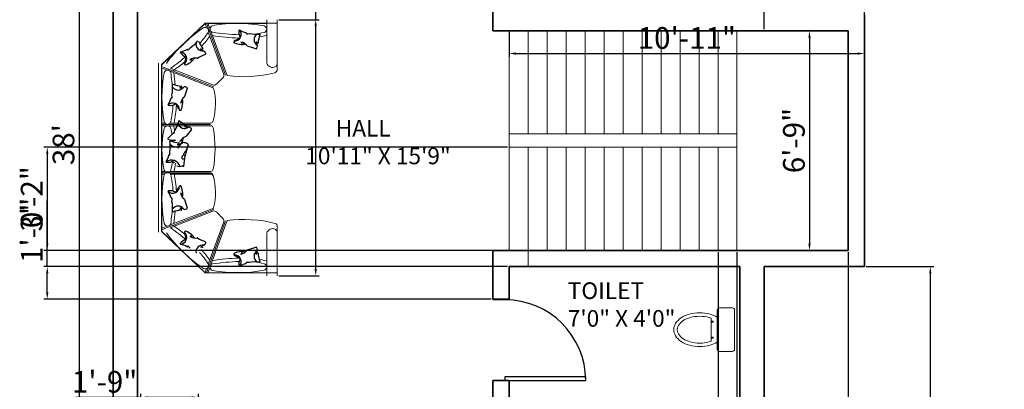
# Model space of a CAD drawing. Units: inches. Extents: x 3064 to 3427, y 2432 to 3115.
# Tile 2 of 3: x 3064 to 3427, y 2696 to 2833. Entities that reach past the tile are written whole.
import ezdxf

# ---------------------------------------------------------------- set-up
doc = ezdxf.new("R2010")
doc.units = ezdxf.units.IN
for name, color, linetype, lineweight in [('A-ANNO-DIMS', 2, 'Continuous', 13), ('A-AREA-IDEN', 7, 'Continuous', 18), ('A-DOOR', 4, 'Continuous', 25), ('A-FLOR-STRS', 3, 'Continuous', 18), ('A-WALL', 7, 'Continuous', 35), ('FUR', 42, 'Continuous', 18), ('THIET-BI', 21, 'Continuous', 18)]:
    doc.layers.add(name, color=color, linetype=linetype, lineweight=lineweight)
doc.layers.add('HID', color=11, linetype='Continuous')
doc.styles.get("Standard").update_dxf_attribs({"font": 'arial.ttf'})
doc.dimstyles.new('ISO-25', dxfattribs={"dimtxt": 8, "dimasz": 2.5, "dimexe": 1.25, "dimexo": 0.625, "dimtad": 1, "dimdec": 0, "dimlunit": 4, "dimtxsty": 'Standard', "dimcen": 2.5, "dimadec": 0, "dimazin": 0, "dimtfac": 1, "dimtdec": 0, "dimtmove": 0, "dimatfit": 3, "dimfxl": 1, "dimarcsym": 0})

# ---------------------------------------------------------------- blocks, each defined once
blk = doc.blocks.new('A$C5B9B1B1E')
at = {"layer": 'FUR'}
for p, q in [((0.68, 1.857), (3.32, 1.857)), ((0.044, 1.127), (0.687, 1.804)), ((0.046, 1.126), (0.691, 1.805)), ((0.687, 1.804), (3.246, 1.804)), ((0.689, 1.807), (3.298, 1.807)), ((0.718, 1.807), (1.035, 0.991)), ((0.741, 1.807), (0.774, 1.719)), ((1.587, 1.804), (1.587, 1.757)), ((1.608, 1.804), (1.608, 1.041)), ((1.629, 1.804), (1.629, 1.757)), ((2.343, 1.804), (2.343, 1.041)), ((2.364, 1.804), (2.364, 1.041)), ((2.385, 1.804), (2.385, 1.757)), ((3.27, 1.807), (2.952, 0.991)), ((3.247, 1.807), (3.213, 1.719)), ((3.942, 1.126), (3.296, 1.805)), ((3.944, 1.127), (3.298, 1.807)), ((0.748, 1.672), (1.007, 1.005)), ((0.792, 1.675), (1.057, 0.993)), ((1.587, 1.671), (1.587, 1.041)), ((1.603, 1.671), (1.603, 1.041)), ((1.629, 1.671), (1.629, 1.041)), ((2.385, 1.671), (2.385, 1.041)), ((3.196, 1.675), (2.93, 0.993)), ((3.24, 1.672), (2.98, 1.005)), ((0.044, 1.127), (0.044, 0)), ((0.044, 1.127), (0.112, 1.103)), ((0.044, 1.105), (0.856, 0.808)), ((0.044, 1.083), (0.133, 1.05)), ((0.046, 1.082), (0.046, 0.164)), ((0.181, 1.077), (0.842, 0.836)), ((3.944, 1.105), (3.131, 0.808)), ((3.807, 1.077), (3.145, 0.836)), ((3.944, 1.083), (3.854, 1.05)), ((3.944, 1.127), (3.875, 1.103)), ((3.941, 1.082), (3.941, 0.164)), ((3.944, 1.127), (3.944, 0)), ((0.167, 1.038), (0.86, 0.785)), ((0.997, 0.952), (0.895, 0.848)), ((2.991, 0.952), (3.093, 0.848)), ((3.82, 1.038), (3.128, 0.785)), ((0, 0.164), (0.663, 0.164)), ((4, 0.164), (3.325, 0.164)), ((0, 0), (0.775, 0)), ((4, 0), (3.219, 0))]:
    blk.add_line(p, q, dxfattribs=at)
for centre, radius, start, end in [((1.999, -0.1), 2.263, 125.9311, 146.4201), ((0.827, 1.714), 0.0525, 104.0803, 255.9197), ((1.2, -0.267), 2.068, 79.3218, 100.7558), ((1.571, 1.714), 0.0529, 283.4421, 76.5579), ((1.661, 1.714), 0.0529, 103.4421, 256.5579), ((1.974, 0.302), 1.499, 77.3591, 102.5496), ((2.289, 1.714), 0.0525, 284.0803, 75.9197), ((2.417, 1.714), 0.0529, 103.4421, 256.5579), ((2.788, -0.267), 2.068, 79.2442, 100.6782), ((3.161, 1.714), 0.0525, 284.0803, 75.9197), ((1.989, -0.1), 2.263, 33.5799, 54.0689), ((-2.245, 3.806), 3.68, 319.5649, 324.3474), ((-2.245, 3.806), 3.733, 320.6889, 324.3474), ((1.373, 5.964), 4.337, 262.5873, 266.2564), ((1.493, 7.461), 5.886, 263.3874, 265.2569), ((1.257, 3.126), 1.499, 272.4014, 282.5496), ((1.257, 3.126), 1.551, 272.4014, 282.5496), ((1.974, 3.126), 1.551, 257.1404, 261.9048), ((1.974, 3.126), 1.499, 257.4504, 262.6454), ((1.974, 3.126), 1.499, 274.5548, 275.3997), ((1.974, 3.126), 1.499, 278.9885, 282.6409), ((1.974, 3.126), 1.551, 280.7847, 283.7486), ((2.73, 3.126), 1.551, 257.4504, 267.5986), ((2.73, 3.126), 1.499, 257.4504, 267.5986), ((2.614, 5.964), 4.337, 273.7436, 277.4127), ((2.494, 7.461), 5.886, 274.7431, 276.6126), ((6.233, 3.806), 3.733, 215.6526, 219.3111), ((6.233, 3.806), 3.68, 215.6526, 220.4351), ((0.159, 1.125), 0.0525, 149.9951, 301.8345), ((-0.635, 2.334), 1.499, 303.2739, 311.5982), ((-0.635, 2.334), 1.551, 304.4606, 312.1941), ((4.623, 2.334), 1.551, 227.8059, 235.5394), ((4.623, 2.334), 1.499, 228.4018, 236.7261), ((3.828, 1.125), 0.0525, 238.1655, 30.0049), ((2.31, 0.617), 2.263, 170.0163, 190.5053), ((0.133, 0.997), 0.0529, 13.4421, 166.5579), ((-3.456, 0.47), 3.68, 1.9572, 8.4326), ((-3.456, 0.47), 3.733, 1.9572, 8.4326), ((0.961, 0.987), 0.05, 315.6002, 21.264), ((1.299, 2.034), 1.068, 256.9274, 284.5801), ((1.545, 1.041), 0.042, 279.7794, 0), ((1.561, 1.041), 0.042, 279.7794, 0), ((1.671, 1.041), 0.042, 180, 260.2206), ((1.986, 2.869), 1.897, 260.2206, 279.7794), ((2.301, 1.041), 0.042, 279.7794, 0), ((2.427, 1.041), 0.042, 180, 260.2206), ((2.689, 2.034), 1.068, 255.4199, 283.0726), ((3.027, 0.987), 0.05, 158.736, 224.3998), ((7.443, 0.47), 3.733, 171.5674, 178.0428), ((7.443, 0.47), 3.68, 171.5674, 178.0428), ((3.854, 0.997), 0.0529, 13.4421, 166.5579), ((1.678, 0.617), 2.263, 349.4947, 9.9837), ((-1.061, 0.519), 1.939, 345.4239, 7.8665), ((0.859, 0.883), 0.05, 249.9365, 315.6002), ((3.128, 0.883), 0.05, 224.3998, 290.0635), ((5.006, 0.521), 1.897, 172.0077, 194.7607), ((-1.275, 0.533), 1.499, 347.3591, 353.601), ((5.263, 0.533), 1.499, 186.399, 192.6409), ((0.136, 0.218), 0.0525, 194.0803, 345.9197), ((-1.275, 0.533), 1.551, 346.2514, 350.7022), ((0.643, 0.074), 0.0918, 328.6411, 77.5888), ((3.345, 0.074), 0.0918, 102.4112, 211.3589), ((5.263, 0.533), 1.551, 189.2978, 193.7486), ((3.851, 0.218), 0.0525, 194.0803, 345.9197), ((0.665, 0.069), 0.0703, 279.5212, 322.6757), ((0.775, 0.042), 0.042, 270, 345.2393), ((3.226, 0.057), 0.0573, 199.356, 262.7582), ((3.338, 0.086), 0.0936, 219.4969, 247.1448)]:
    blk.add_arc(centre, radius, start, end, dxfattribs=at)
at = {"layer": 'HID'}
for centre, radius, start, end in [((1.056, 2.162), 0.527, 287.478, 299.4698), ((1.393, 1.632), 0.104, 135.6927, 273.5175), ((1.159, 1.674), 0.168, 330.4242, 8.3824), ((1.319, 1.698), 0.0063, 8.3824, 119.4698), ((1.664, 1.652), 0.142, 287.6048, 36.1053), ((1.94, 1.709), 0.168, 172.876, 210.0789), ((1.78, 1.729), 0.0063, 61.7886, 172.876), ((1.78, 1.729), 0.0063, 61.7886, 172.876), ((2.032, 2.199), 0.527, 241.7886, 253.7804), ((1.883, 1.687), 0.0063, 339.311, 73.7804), ((2.283, 1.626), 0.168, 151.6176, 189.5758), ((2.141, 1.703), 0.0063, 40.5302, 151.6176), ((2.546, 2.05), 0.527, 220.5302, 232.522), ((2.594, 1.632), 0.104, 266.4825, 44.3073), ((2.829, 1.674), 0.168, 171.6176, 209.5758), ((2.669, 1.698), 0.0063, 60.5302, 171.6176), ((2.931, 2.162), 0.527, 240.5302, 252.522), ((1, 1.632), 0.0063, 83.9832, 202.2174), ((0.606, 1.471), 0.42, 3.9947, 22.2174), ((1.056, 2.162), 0.527, 263.9832, 281.5286), ((0.982, 1.549), 0.105, 304.0212, 55.1506), ((1.202, 1.894), 0.252, 260.6752, 270.5669), ((1.205, 1.649), 0.0063, 270.5669, 21.9475), ((1.216, 1.653), 0.0063, 107.478, 201.9475), ((1.31, 1.588), 0.0063, 150.4242, 237.1103), ((1.981, 2.625), 1.241, 237.1103, 241.1368), ((1.379, 1.514), 0.0244, 343.8009, 85.0524), ((1.809, 1.522), 0.102, 154.2387, 202.8337), ((1.795, 1.618), 0.0252, 110.8427, 217.338), ((1.859, 0.222), 1.409, 92.7112, 93.5018), ((2.33, 2.894), 1.409, 247.2794, 247.2982), ((1.791, 1.62), 0.0063, 304.1671, 51.1685), ((1.895, 1.683), 0.0063, 159.311, 270.6915), ((1.892, 1.928), 0.252, 270.6915, 280.5832), ((2.032, 2.199), 0.527, 259.7298, 277.2752), ((2.009, 1.552), 0.0126, 176.1991, 230.6607), ((2.302, 1.91), 0.476, 230.6607, 243.8744), ((2.119, 1.588), 0.105, 126.1078, 237.2372), ((2.088, 1.569), 0.0416, 194.2109, 241.7015), ((2.179, 1.559), 0.131, 180.2155, 218.3929), ((2.072, 1.538), 0.0063, 241.7015, 357.2637), ((2.497, 1.518), 0.42, 159.041, 177.2637), ((2.099, 1.67), 0.0063, 339.041, 97.2752), ((2.111, 1.597), 0.0063, 282.8897, 9.5758), ((2.231, 1.618), 0.0063, 138.0525, 249.4331), ((2.222, 1.627), 0.0063, 318.0525, 52.522), ((2.317, 1.848), 0.252, 249.4331, 259.3248), ((2.546, 2.05), 0.527, 238.4714, 256.0168), ((2.406, 1.449), 0.105, 104.8494, 215.9788), ((2.417, 1.532), 0.0063, 317.7826, 76.0168), ((2.608, 1.514), 0.0244, 94.9476, 196.1991), ((2.007, 2.625), 1.241, 298.8632, 302.8897), ((2.677, 1.588), 0.0063, 302.8897, 29.5758), ((2.771, 1.653), 0.0063, 338.0525, 72.522), ((2.783, 1.649), 0.0063, 158.0525, 269.4331), ((2.785, 1.894), 0.252, 269.4331, 279.3248), ((2.931, 2.162), 0.527, 258.4714, 276.0168), ((3.005, 1.549), 0.105, 124.8494, 235.9788), ((3.382, 1.471), 0.42, 157.7826, 176.0053), ((2.987, 1.632), 0.0063, 337.7826, 96.0168), ((0.277, 1.564), 0.252, 306.59, 316.4817), ((0.459, 1.407), 0.0063, 153.3928, 247.8623), ((-0.018, 1.646), 0.527, 333.3928, 345.3846), ((0.455, 1.395), 0.0063, 316.4817, 67.8623), ((0.498, 1.511), 0.0063, 54.2972, 165.3846), ((0.598, 1.519), 0.104, 181.6075, 319.4323), ((0.404, 1.38), 0.168, 16.339, 54.2972), ((0.571, 1.429), 0.0063, 196.339, 283.0251), ((0.293, 2.632), 1.241, 283.0251, 287.0516), ((0.263, 1.627), 0.476, 322.0404, 335.2541), ((0.673, 1.427), 0.0244, 29.7157, 130.9672), ((0.683, 1.433), 0.0126, 335.2541, 29.7157), ((1.031, 1.5), 0.0063, 183.9947, 299.557), ((1.013, 1.531), 0.0416, 299.557, 347.0475), ((0.923, 1.519), 0.131, 329.5087, 1.0429), ((1.135, 1.458), 0.099, 182.7962, 207.1304), ((1.058, 1.418), 0.0126, 207.1304, 290.9482), ((1.531, 0.183), 1.31, 105.1521, 110.9482), ((1.185, 1.46), 0.0126, 285.1521, 322.4345), ((1.324, 1.352), 0.163, 100.921, 142.4345), ((1.274, 1.728), 0.252, 258.5381, 270.9308), ((1.286, 1.487), 0.0126, 131.4659, 280.4525), ((1.185, 1.602), 0.141, 311.4659, 320.8131), ((1.237, 1.948), 0.476, 276.1256, 289.3393), ((1.391, 1.511), 0.0126, 289.3393, 343.8009), ((1.704, 1.478), 0.0126, 265.6578, 22.8337), ((1.603, 0.159), 1.31, 70.5535, 85.4148), ((1.85, 1.466), 0.0267, 24.2238, 217.6435), ((1.852, 1.466), 0.0279, 302.8444, 337.2985), ((1.866, 1.46), 0.0126, 337.2985, 347.3574), ((1.891, 1.454), 0.0126, 60.951, 167.3574), ((1.614, 0.955), 0.583, 52.6177, 60.951), ((1.977, 1.428), 0.0126, 226.2045, 253.614), ((1.603, 0.159), 1.31, 70.5535, 73.614), ((2.044, 1.406), 0.0126, 250.5535, 318.334), ((1.976, 1.466), 0.103, 318.334, 2.6623), ((2.067, 1.47), 0.0126, 2.6623, 38.3929), ((2.099, 1.494), 0.0126, 239.5475, 28.5341), ((2.234, 1.567), 0.141, 199.1869, 208.5341), ((2.017, 1.381), 0.163, 17.5655, 59.079), ((2.193, 1.717), 0.252, 249.0692, 261.4619), ((2.185, 1.434), 0.0126, 197.5655, 234.8479), ((1.423, 0.352), 1.31, 49.0518, 54.8479), ((2.452, 1.4), 0.131, 158.9571, 190.4913), ((2.371, 1.442), 0.0416, 172.9525, 220.443), ((2.344, 1.419), 0.0063, 220.443, 336.0053), ((2.733, 1.246), 0.42, 137.7826, 156.0053), ((2.597, 1.511), 0.0126, 196.1991, 250.6607), ((2.75, 1.948), 0.476, 250.6607, 263.8744), ((2.663, 1.352), 0.163, 37.5655, 79.079), ((2.803, 1.602), 0.141, 219.1869, 228.5341), ((2.702, 1.487), 0.0126, 259.5475, 48.5341), ((2.713, 1.728), 0.252, 269.0692, 281.4619), ((2.803, 1.46), 0.0126, 217.5655, 254.8479), ((2.457, 0.183), 1.31, 69.0518, 74.8479), ((2.93, 1.418), 0.0126, 249.0518, 332.8696), ((3.065, 1.519), 0.131, 178.9571, 210.4913), ((2.974, 1.531), 0.0416, 192.9525, 240.443), ((2.853, 1.458), 0.099, 332.8696, 357.2038), ((2.957, 1.5), 0.0063, 240.443, 356.0053), ((3.304, 1.433), 0.0126, 150.2843, 204.7459), ((3.315, 1.427), 0.0244, 49.0328, 150.2843), ((3.725, 1.627), 0.476, 204.7459, 217.9596), ((3.389, 1.519), 0.104, 220.5677, 358.3925), ((3.694, 2.632), 1.241, 252.9484, 256.9749), ((3.416, 1.429), 0.0063, 256.9749, 343.661), ((3.583, 1.38), 0.168, 125.7028, 163.661), ((4.005, 1.646), 0.527, 194.6154, 206.6072), ((3.533, 1.395), 0.0063, 112.1377, 223.5183), ((3.711, 1.564), 0.252, 223.5183, 233.41), ((3.528, 1.407), 0.0063, 292.1377, 26.6072), ((0.371, 1.166), 0.105, 349.936, 101.0654), ((1.734, 0.609), 1.31, 151.0669, 156.863), ((0.751, 1.275), 0.163, 146.8358, 188.3493), ((0.446, 1.501), 0.252, 304.4529, 316.8456), ((0.577, 1.249), 0.0126, 331.0669, 8.3493), ((0.474, 1.348), 0.141, 357.3807, 6.7279), ((0.627, 1.341), 0.0126, 177.3807, 326.3673), ((2.29, 1.351), 0.0126, 229.0518, 312.8696), ((2.232, 1.415), 0.099, 312.8696, 337.2038), ((3.36, 1.341), 0.0126, 213.6327, 2.6193), ((3.542, 1.501), 0.252, 223.1544, 235.5471), ((3.513, 1.348), 0.141, 173.2721, 182.6193), ((3.237, 1.275), 0.163, 351.6507, 33.1642), ((3.411, 1.249), 0.0126, 171.6507, 208.9331), ((2.253, 0.609), 1.31, 23.137, 28.9331), ((3.616, 1.166), 0.105, 78.9346, 190.064), ((3.822, 0.841), 0.42, 111.8678, 130.0905), ((4.005, 1.646), 0.527, 212.5566, 230.102), ((0.44, 1.167), 0.0063, 229.9095, 345.4718), ((0.406, 1.176), 0.0416, 345.4718, 32.9623), ((0.351, 1.103), 0.131, 15.4235, 46.9577), ((0.543, 1.212), 0.099, 228.711, 253.0452), ((0.518, 1.129), 0.0126, 253.0452, 336.863), ((3.47, 1.129), 0.0126, 203.137, 286.9548), ((3.445, 1.212), 0.099, 286.9548, 311.289), ((3.636, 1.103), 0.131, 133.0423, 164.5765), ((3.582, 1.176), 0.0416, 147.0377, 194.5282), ((3.547, 1.167), 0.0063, 194.5282, 310.0905), ((0.219, 0.669), 0.104, 225.6927, 3.5175), ((-0.775, 1.256), 1.241, 327.1103, 331.1368), ((0.336, 0.655), 0.0244, 73.8009, 175.0524), ((0.34, 0.666), 0.0126, 19.3393, 73.8009), ((-0.097, 0.513), 0.476, 6.1256, 19.3393), ((4.085, 0.513), 0.476, 160.6607, 173.8744), ((3.648, 0.666), 0.0126, 106.1991, 160.6607), ((3.651, 0.655), 0.0244, 4.9476, 106.1991), ((3.769, 0.669), 0.104, 176.4825, 314.3073), ((4.762, 1.256), 1.241, 208.8632, 212.8897), ((0.152, 0.594), 0.0063, 98.3824, 209.4698), ((-0.312, 0.331), 0.527, 17.478, 29.4698), ((0.176, 0.434), 0.168, 60.4242, 98.3824), ((0.197, 0.492), 0.0063, 197.478, 291.9475), ((0.202, 0.48), 0.0063, 0.5669, 111.9475), ((-0.044, 0.478), 0.252, 350.6752, 0.5669), ((0.262, 0.586), 0.0063, 240.4242, 327.1103), ((0.498, 0.6), 0.163, 190.921, 232.4345), ((0.249, 0.46), 0.141, 41.4659, 50.8131), ((0.363, 0.561), 0.0126, 221.4659, 10.4525), ((0.122, 0.55), 0.252, 348.5381, 0.9308), ((0.391, 0.46), 0.0126, 15.1521, 52.4345), ((1.668, 0.806), 1.31, 195.1521, 200.9482), ((2.32, 0.806), 1.31, 339.0518, 344.8479), ((3.597, 0.46), 0.0126, 127.5655, 164.8479), ((3.49, 0.6), 0.163, 307.5655, 349.079), ((3.624, 0.561), 0.0126, 169.5475, 318.5341), ((3.866, 0.55), 0.252, 179.0692, 191.4619), ((3.739, 0.46), 0.141, 129.1869, 138.5341), ((3.726, 0.586), 0.0063, 212.8897, 299.5758), ((3.811, 0.434), 0.168, 81.6176, 119.5758), ((3.786, 0.48), 0.0063, 68.0525, 179.4331), ((4.031, 0.478), 0.252, 179.4331, 189.3248), ((3.791, 0.492), 0.0063, 248.0525, 342.522), ((4.3, 0.331), 0.527, 150.5302, 162.522), ((-0.312, 0.331), 0.527, 353.9832, 11.5286), ((0.301, 0.258), 0.105, 34.0212, 145.1506), ((0.319, 0.289), 0.0416, 29.557, 77.0475), ((0.331, 0.198), 0.131, 59.5087, 91.0429), ((0.35, 0.306), 0.0063, 273.9947, 29.557), ((0.393, 0.41), 0.099, 272.7962, 297.1304), ((0.432, 0.333), 0.0126, 297.1304, 20.9482), ((3.556, 0.333), 0.0126, 159.0518, 242.8696), ((3.595, 0.41), 0.099, 242.8696, 267.2038), ((3.657, 0.198), 0.131, 88.9571, 120.4913), ((3.687, 0.258), 0.105, 34.8494, 145.9788), ((3.638, 0.306), 0.0063, 150.443, 266.0053), ((3.668, 0.289), 0.0416, 102.9525, 150.443), ((4.3, 0.331), 0.527, 168.4714, 186.0168), ((0.219, 0.276), 0.0063, 173.9832, 292.2174), ((0.38, -0.119), 0.42, 93.9947, 112.2174), ((3.608, -0.119), 0.42, 67.7826, 86.0053), ((3.769, 0.276), 0.0063, 247.7826, 6.0168)]:
    blk.add_arc(centre, radius, start, end, dxfattribs=at)
blk = doc.blocks.new('*D6')
at = {"layer": 'A-ANNO-DIMS', "color": 0, "lineweight": -2, "transparency": 16777216}
for p, q in [((3338.05, 2829.08), (3338.05, 2839.48)), ((3375.05, 2829.08), (3375.05, 2839.48)), ((3340.55, 2838.23), (3372.55, 2838.23))]:
    blk.add_line(p, q, dxfattribs=at)
at = {"layer": 'A-ANNO-DIMS', "color": 0, "transparency": 16777216}
for points in [[(3340.55, 2838.65), (3340.55, 2837.82), (3338.05, 2838.23)], [(3372.55, 2838.65), (3372.55, 2837.82), (3375.05, 2838.23)]]:
    blk.add_solid(points, dxfattribs=at)
at = {"layer": 'Defpoints', "color": 0, "transparency": 16777216}
for p in [(3375.05, 2838.23), (3338.05, 2828.45), (3375.05, 2828.45)]:
    blk.add_point(p, dxfattribs=at)
at = {"layer": 'A-ANNO-DIMS', "color": 0, "transparency": 16777216, "insert": (3356.55, 2842.95), "char_height": 8, "attachment_point": 5}
blk.add_mtext('3\'-1"', dxfattribs=at)
blk = doc.blocks.new('*D7')
at = {"layer": 'A-ANNO-DIMS', "color": 0, "lineweight": -2, "transparency": 16777216}
for p, q in [((3244.05, 2827.83), (3244.05, 2818.79)), ((3375.05, 2827.83), (3375.05, 2818.79)), ((3246.55, 2820.04), (3372.55, 2820.04))]:
    blk.add_line(p, q, dxfattribs=at)
at = {"layer": 'A-ANNO-DIMS', "color": 0, "transparency": 16777216}
for points in [[(3246.55, 2820.45), (3246.55, 2819.62), (3244.05, 2820.04)], [(3372.55, 2820.45), (3372.55, 2819.62), (3375.05, 2820.04)]]:
    blk.add_solid(points, dxfattribs=at)
at = {"layer": 'Defpoints', "color": 0, "transparency": 16777216}
for p in [(3244.05, 2828.45), (3375.05, 2828.45), (3375.05, 2820.04)]:
    blk.add_point(p, dxfattribs=at)
at = {"layer": 'A-ANNO-DIMS', "color": 0, "transparency": 16777216, "insert": (3309.55, 2824.75), "char_height": 8, "attachment_point": 5}
blk.add_mtext('10\'-11"', dxfattribs=at)
blk = doc.blocks.new('*D8')
at = {"layer": 'A-ANNO-DIMS', "color": 0, "lineweight": -2, "transparency": 16777216}
for p, q in [((3368.42, 2828.45), (3353.52, 2828.45)), ((3354.77, 2825.95), (3354.77, 2749.95)), ((3368.42, 2747.45), (3353.52, 2747.45))]:
    blk.add_line(p, q, dxfattribs=at)
at = {"layer": 'A-ANNO-DIMS', "color": 0, "transparency": 16777216}
for points in [[(3354.35, 2825.95), (3355.19, 2825.95), (3354.77, 2828.45)], [(3354.35, 2749.95), (3355.19, 2749.95), (3354.77, 2747.45)]]:
    blk.add_solid(points, dxfattribs=at)
at = {"layer": 'Defpoints', "color": 0, "transparency": 16777216}
for p in [(3369.05, 2828.45), (3354.77, 2747.45), (3369.05, 2747.45)]:
    blk.add_point(p, dxfattribs=at)
at = {"layer": 'A-ANNO-DIMS', "color": 0, "transparency": 16777216, "insert": (3350.06, 2787.95), "char_height": 8, "attachment_point": 5, "rotation": 90}
blk.add_mtext('6\'-9"', dxfattribs=at)
blk = doc.blocks.new('*U13')
for p, q in [((0, 0), (0, 6)), ((40, 0), (40, 6))]:
    blk.add_line(p, q)
blk.add_lwpolyline([(0, 0), (0, -40), (1.75, -40), (1.75, 0)], close=True)
blk.add_arc((0, 0), 40, 270, 360)
blk = doc.blocks.new('*D16')
at = {"layer": 'A-ANNO-DIMS', "color": 0, "lineweight": -2, "transparency": 16777216}
for p, q in [((3097.42, 3014.45), (3084.25, 3014.45)), ((3085.5, 3011.95), (3085.5, 2560.95)), ((3097.42, 2558.45), (3084.25, 2558.45))]:
    blk.add_line(p, q, dxfattribs=at)
at = {"layer": 'A-ANNO-DIMS', "color": 0, "transparency": 16777216}
for points in [[(3085.09, 3011.95), (3085.92, 3011.95), (3085.5, 3014.45)], [(3085.09, 2560.95), (3085.92, 2560.95), (3085.5, 2558.45)]]:
    blk.add_solid(points, dxfattribs=at)
at = {"layer": 'Defpoints', "color": 0, "transparency": 16777216}
for p in [(3098.05, 3014.45), (3085.5, 2558.45), (3098.05, 2558.45)]:
    blk.add_point(p, dxfattribs=at)
at = {"layer": 'A-ANNO-DIMS', "color": 0, "transparency": 16777216, "insert": (3080.79, 2786.45), "char_height": 8, "attachment_point": 5, "rotation": 90}
blk.add_mtext("38'", dxfattribs=at)
blk = doc.blocks.new('WC-TANK')
for p, q in [((16.04, 15.24), (16.04, 0.8)), ((21.66, 16.04), (16.85, 16.04)), ((22.46, 0.8), (22.46, 15.24)), ((13.79, 11.11), (13.79, 10.8)), ((14.52, 11.11), (13.79, 11.11)), ((13.8, 12.29), (13.8, 3.76)), ((14.52, 10.8), (14.52, 11.11)), ((13.79, 10.8), (14.52, 10.8)), ((13.79, 4.94), (13.79, 5.26)), ((13.79, 5.26), (14.52, 5.26)), ((14.52, 4.94), (13.79, 4.94)), ((14.52, 5.26), (14.52, 4.94)), ((16.85, 0), (21.66, 0))]:
    blk.add_line(p, q)
for centre, radius, start, end in [((16.85, 15.24), 0.802, 90, 180), ((21.66, 15.24), 0.802, 0, 90), ((6.75, 6.36), 7.24, 123.0315, 147.5002), ((6.75, 6.36), 5.95, 123.0315, 147.5002), ((8.47, 3.73), 10.38, 105.0731, 123.0315), ((8.47, 3.73), 9.1, 105.0731, 123.0315), ((9.59, -0.44), 14.7, 74.9269, 105.0732), ((9.59, -0.44), 13.41, 74.9269, 105.0732), ((10.71, 3.73), 9.1, 70.176, 74.9269), ((10.71, 3.73), 10.38, 59.0966, 74.9269), ((4.15, 8.02), 4.15, 147.5002, 212.4998), ((4.15, 8.02), 2.87, 147.5002, 212.4998), ((6.75, 9.68), 7.24, 212.4998, 236.9685), ((6.75, 9.68), 5.95, 212.4998, 236.9685), ((8.47, 12.31), 9.1, 236.9685, 254.9269), ((10.71, 12.31), 9.1, 285.0731, 289.824), ((8.47, 12.31), 10.38, 236.9685, 254.9269), ((9.59, 16.48), 14.7, 254.9269, 285.0731), ((9.59, 16.48), 13.41, 254.9269, 285.0731), ((10.71, 12.31), 10.38, 285.0731, 300.9034), ((16.85, 0.8), 0.802, 180, 270), ((21.66, 0.8), 0.802, 270, 0)]:
    blk.add_arc(centre, radius, start, end)
blk = doc.blocks.new('*D23')
at = {"layer": 'A-ANNO-DIMS', "color": 0, "lineweight": -2, "transparency": 16777216}
for p, q in [((3108.3, 2686.11), (3108.3, 2694.47)), ((3129.5, 2686.11), (3129.5, 2694.47)), ((3108.3, 2693.22), (3084.03, 2693.22)), ((3127, 2693.22), (3110.8, 2693.22))]:
    blk.add_line(p, q, dxfattribs=at)
at = {"layer": 'A-ANNO-DIMS', "color": 0, "transparency": 16777216}
for points in [[(3110.8, 2693.64), (3110.8, 2692.81), (3108.3, 2693.22)], [(3127, 2693.64), (3127, 2692.81), (3129.5, 2693.22)]]:
    blk.add_solid(points, dxfattribs=at)
at = {"layer": 'Defpoints', "color": 0, "transparency": 16777216}
for p in [(3108.3, 2693.22), (3108.3, 2685.48), (3129.5, 2685.48)]:
    blk.add_point(p, dxfattribs=at)
at = {"layer": 'A-ANNO-DIMS', "color": 0, "transparency": 16777216, "insert": (3094.91, 2697.93), "char_height": 8, "attachment_point": 5}
blk.add_mtext('1\'-9"', dxfattribs=at)
blk = doc.blocks.new('*D24')
at = {"layer": 'A-ANNO-DIMS', "color": 0, "lineweight": -2, "transparency": 16777216}
for p, q in [((3304.5, 2851.35), (3304.5, 2847.32)), ((3327.18, 2851.35), (3327.18, 2847.32)), ((3307, 2848.57), (3324.68, 2848.57)), ((3327.18, 2848.57), (3426.6, 2848.57))]:
    blk.add_line(p, q, dxfattribs=at)
at = {"layer": 'A-ANNO-DIMS', "color": 0, "transparency": 16777216}
for points in [[(3307, 2848.99), (3307, 2848.15), (3304.5, 2848.57)], [(3324.68, 2848.99), (3324.68, 2848.15), (3327.18, 2848.57)]]:
    blk.add_solid(points, dxfattribs=at)
at = {"layer": 'Defpoints', "color": 0, "transparency": 16777216}
for p in [(3304.5, 2851.97), (3327.18, 2851.97), (3327.18, 2848.57)]:
    blk.add_point(p, dxfattribs=at)
at = {"layer": 'A-ANNO-DIMS', "color": 0, "transparency": 16777216, "insert": (3378.14, 2853.33), "char_height": 8, "attachment_point": 5}
blk.add_mtext('WC 1\'-10 1/2" TYP.', dxfattribs=at)
blk = doc.blocks.new('*D28')
at = {"layer": 'A-ANNO-DIMS', "color": 0, "lineweight": -2, "transparency": 16777216}
for p, q in [((3172.73, 2832.53), (3172.73, 2982.35)), ((3159.19, 2832.53), (3173.98, 2832.53)), ((3172.73, 2740.61), (3172.73, 2830.03)), ((3159.19, 2738.11), (3173.98, 2738.11))]:
    blk.add_line(p, q, dxfattribs=at)
at = {"layer": 'A-ANNO-DIMS', "color": 0, "transparency": 16777216}
for points in [[(3172.31, 2830.03), (3173.15, 2830.03), (3172.73, 2832.53)], [(3172.31, 2740.61), (3173.15, 2740.61), (3172.73, 2738.11)]]:
    blk.add_solid(points, dxfattribs=at)
at = {"layer": 'Defpoints', "color": 0, "transparency": 16777216}
for p in [(3158.57, 2832.53), (3172.73, 2832.53), (3158.57, 2738.11)]:
    blk.add_point(p, dxfattribs=at)
at = {"layer": 'A-ANNO-DIMS', "color": 0, "transparency": 16777216, "insert": (3167.96, 2908.69), "char_height": 8, "attachment_point": 5, "rotation": 90}
blk.add_mtext('SECTIONAL SOFA 7\'-10 1/2"', dxfattribs=at)
blk = doc.blocks.new('*D36')
at = {"layer": 'A-ANNO-DIMS', "color": 0, "lineweight": -2, "transparency": 16777216}
for p, q in [((3375.67, 2741.45), (3400.58, 2741.45)), ((3399.33, 2560.95), (3399.33, 2738.95)), ((3338.67, 2558.45), (3400.58, 2558.45))]:
    blk.add_line(p, q, dxfattribs=at)
at = {"layer": 'A-ANNO-DIMS', "color": 0, "transparency": 16777216}
for points in [[(3398.91, 2738.95), (3399.74, 2738.95), (3399.33, 2741.45)], [(3398.91, 2560.95), (3399.74, 2560.95), (3399.33, 2558.45)]]:
    blk.add_solid(points, dxfattribs=at)
at = {"layer": 'Defpoints', "color": 0, "transparency": 16777216}
for p in [(3375.05, 2741.45), (3399.33, 2741.45), (3338.05, 2558.45)]:
    blk.add_point(p, dxfattribs=at)
at = {"layer": 'A-ANNO-DIMS', "color": 0, "transparency": 16777216, "insert": (3394.61, 2649.95), "char_height": 8, "attachment_point": 5, "rotation": 90}
blk.add_mtext('15\'-3"', dxfattribs=at)
blk = doc.blocks.new('*D37')
at = {"layer": 'A-ANNO-DIMS', "color": 0, "lineweight": -2, "transparency": 16777216}
for p, q in [((3328.05, 2746.83), (3328.05, 2532.92)), ((3369.05, 2746.83), (3369.05, 2532.92)), ((3330.55, 2534.17), (3366.55, 2534.17))]:
    blk.add_line(p, q, dxfattribs=at)
at = {"layer": 'A-ANNO-DIMS', "color": 0, "transparency": 16777216}
for points in [[(3330.55, 2534.59), (3330.55, 2533.75), (3328.05, 2534.17)], [(3366.55, 2534.59), (3366.55, 2533.75), (3369.05, 2534.17)]]:
    blk.add_solid(points, dxfattribs=at)
at = {"layer": 'Defpoints', "color": 0, "transparency": 16777216}
for p in [(3328.05, 2747.45), (3369.05, 2747.45), (3369.05, 2534.17)]:
    blk.add_point(p, dxfattribs=at)
at = {"layer": 'A-ANNO-DIMS', "color": 0, "transparency": 16777216, "insert": (3348.55, 2538.88), "char_height": 8, "attachment_point": 5}
blk.add_mtext('3\'-5"', dxfattribs=at)
blk = doc.blocks.new('*D38')
at = {"layer": 'A-ANNO-DIMS', "color": 0, "lineweight": -2, "transparency": 16777216}
for p, q in [((3321.05, 2746.83), (3321.05, 2532.92)), ((3328.05, 2746.83), (3328.05, 2532.92)), ((3323.55, 2534.17), (3325.55, 2534.17)), ((3328.05, 2534.17), (3353.06, 2534.17))]:
    blk.add_line(p, q, dxfattribs=at)
at = {"layer": 'A-ANNO-DIMS', "color": 0, "transparency": 16777216}
for points in [[(3323.55, 2534.59), (3323.55, 2533.75), (3321.05, 2534.17)], [(3325.55, 2534.59), (3325.55, 2533.75), (3328.05, 2534.17)]]:
    blk.add_solid(points, dxfattribs=at)
at = {"layer": 'Defpoints', "color": 0, "transparency": 16777216}
for p in [(3321.05, 2747.45), (3328.05, 2747.45), (3328.05, 2534.17)]:
    blk.add_point(p, dxfattribs=at)
at = {"layer": 'A-ANNO-DIMS', "color": 0, "transparency": 16777216, "insert": (3341.8, 2538.88), "char_height": 8, "attachment_point": 5}
blk.add_mtext('0\'-7"', dxfattribs=at)
blk = doc.blocks.new('*D39')
at = {"layer": 'A-ANNO-DIMS', "color": 0, "lineweight": -2, "transparency": 16777216}
for p, q in [((3243.42, 2785.45), (3072.52, 2785.45)), ((3073.77, 2782.95), (3073.77, 2749.95)), ((3243.42, 2747.45), (3072.52, 2747.45))]:
    blk.add_line(p, q, dxfattribs=at)
at = {"layer": 'A-ANNO-DIMS', "color": 0, "transparency": 16777216}
for points in [[(3073.35, 2782.95), (3074.18, 2782.95), (3073.77, 2785.45)], [(3073.35, 2749.95), (3074.18, 2749.95), (3073.77, 2747.45)]]:
    blk.add_solid(points, dxfattribs=at)
at = {"layer": 'Defpoints', "color": 0, "transparency": 16777216}
for p in [(3244.05, 2785.45), (3073.77, 2747.45), (3244.05, 2747.45)]:
    blk.add_point(p, dxfattribs=at)
at = {"layer": 'A-ANNO-DIMS', "color": 0, "transparency": 16777216, "insert": (3069.05, 2766.45), "char_height": 8, "attachment_point": 5, "rotation": 90}
blk.add_mtext('3\'-2"', dxfattribs=at)
blk = doc.blocks.new('*D42')
at = {"layer": 'A-ANNO-DIMS', "color": 0, "lineweight": -2, "transparency": 16777216}
for p, q in [((3073.77, 2741.45), (3073.77, 2765.71)), ((3243.42, 2741.45), (3072.52, 2741.45)), ((3073.77, 2731.95), (3073.77, 2738.95)), ((3237.42, 2729.45), (3072.52, 2729.45))]:
    blk.add_line(p, q, dxfattribs=at)
at = {"layer": 'A-ANNO-DIMS', "color": 0, "transparency": 16777216}
for points in [[(3073.35, 2738.95), (3074.18, 2738.95), (3073.77, 2741.45)], [(3073.35, 2731.95), (3074.18, 2731.95), (3073.77, 2729.45)]]:
    blk.add_solid(points, dxfattribs=at)
at = {"layer": 'Defpoints', "color": 0, "transparency": 16777216}
for p in [(3073.77, 2741.45), (3244.05, 2741.45), (3238.05, 2729.45)]:
    blk.add_point(p, dxfattribs=at)
at = {"layer": 'A-ANNO-DIMS', "color": 0, "transparency": 16777216, "insert": (3069.06, 2754.83), "char_height": 8, "attachment_point": 5, "rotation": 90}
blk.add_mtext('1\'-0"', dxfattribs=at)

msp = doc.modelspace()

# ---------------------------------------------------------------- linework, layer by layer
at = {"layer": 'A-FLOR-STRS'}
for p, q in [((3244.05, 2747.45), (3244.05, 2828.45)), ((3251.05, 2790.45), (3251.05, 2828.45)), ((3258.05, 2790.45), (3258.05, 2828.45)), ((3265.05, 2790.45), (3265.05, 2828.45)), ((3272.05, 2790.45), (3272.05, 2828.45)), ((3279.05, 2790.45), (3279.05, 2828.45)), ((3286.05, 2790.45), (3286.05, 2828.45)), ((3293.05, 2790.45), (3293.05, 2828.45)), ((3300.05, 2790.45), (3300.05, 2828.45)), ((3307.05, 2790.45), (3307.05, 2828.45)), ((3314.05, 2790.45), (3314.05, 2828.45)), ((3321.05, 2790.45), (3321.05, 2828.45)), ((3328.05, 2747.45), (3328.05, 2828.45)), ((3244.05, 2790.45), (3328.05, 2790.45)), ((3244.05, 2785.45), (3328.05, 2785.45)), ((3251.05, 2741.45), (3251.05, 2785.45)), ((3258.05, 2747.45), (3258.05, 2785.45)), ((3265.05, 2747.45), (3265.05, 2785.45)), ((3272.05, 2747.45), (3272.05, 2785.45)), ((3279.05, 2747.45), (3279.05, 2785.45)), ((3286.05, 2747.45), (3286.05, 2785.45)), ((3293.05, 2747.45), (3293.05, 2785.45)), ((3300.05, 2747.45), (3300.05, 2785.45)), ((3307.05, 2747.45), (3307.05, 2785.45)), ((3314.05, 2747.45), (3314.05, 2785.45)), ((3321.05, 2747.45), (3321.05, 2785.45))]:
    msp.add_line(p, q, dxfattribs=at)
at = {"layer": 'A-WALL'}
for p, q in [((3098.05, 2558.45), (3098.05, 3014.45)), ((3107.05, 2693.45), (3107.05, 2882.45)), ((3238.05, 2828.45), (3238.05, 2846.45)), ((3375.05, 2834.28), (3375.05, 2828.45)), ((3238.05, 2828.45), (3338.05, 2828.45)), ((3338.05, 2828.45), (3369.05, 2828.45)), ((3369.05, 2828.45), (3369.05, 2747.45)), ((3375.05, 2828.45), (3375.05, 2747.45)), ((3238.05, 2747.45), (3369.05, 2747.45)), ((3238.05, 2729.45), (3238.05, 2747.45)), ((3375.05, 2741.45), (3375.05, 2747.45)), ((3244.05, 2741.45), (3329.05, 2741.45)), ((3244.05, 2729.45), (3244.05, 2741.45)), ((3329.05, 2741.45), (3329.05, 2693.45)), ((3338.05, 2741.45), (3338.05, 2558.45)), ((3338.05, 2741.45), (3375.05, 2741.45)), ((3238.05, 2729.45), (3244.05, 2729.45)), ((3238.05, 2693.45), (3238.05, 2699.45)), ((3238.05, 2699.45), (3244.05, 2699.45)), ((3244.05, 2693.45), (3244.05, 2699.45))]:
    msp.add_line(p, q, dxfattribs=at)

# ---------------------------------------------------------------- block references
at = {"layer": 'A-DOOR', "xscale": 0.744170698258995, "yscale": 0.744170698258995, "zscale": 0.744170698258995, "rotation": 90}
msp.add_blockref('*U13', (3242.51, 2699.45), dxfattribs=at)
at = {"layer": 'FUR', "xscale": 23.60535253345627, "yscale": 23.60535253345627, "zscale": 23.60535253345627, "rotation": 90}
msp.add_blockref('A$C5B9B1B1E', (3158.57, 2738.11), dxfattribs=at)
at = {"layer": 'THIET-BI'}
msp.add_blockref('WC-TANK', (3304.71, 2710.17), dxfattribs=at)

# ---------------------------------------------------------------- texts
at = {"layer": 'A-AREA-IDEN', "char_height": 6.1325, "attachment_point": 1}
for s, insert in [('      HALL\\P10\'11" X 15\'9"', (3168.88, 2795.57)), ('TOILET\\P7\'0" X 4\'0"', (3265.65, 2735.64))]:
    msp.add_mtext_dynamic_manual_height_columns(s, width=649.6086, gutter_width=30.66, heights=[0], dxfattribs=dict(at, insert=insert))

# ---------------------------------------------------------------- dimensions: what is measured, and where the dimension line sits
at = {"layer": 'A-ANNO-DIMS'}
for base, p1, p2, angle, override, picture, middle in [((3085.5, 2558.45), (3098.05, 3014.45), (3098.05, 2558.45), 90, {"dimclrd": 0, "dimclre": 0, "dimclrt": 0}, '*D16', (3080.79, 2786.45)), ((3354.77, 2747.45), (3369.05, 2828.45), (3369.05, 2747.45), 90, {"dimclrd": 0, "dimclre": 0, "dimclrt": 0}, '*D8', (3350.06, 2787.95)), ((3073.77, 2747.45), (3244.05, 2785.45), (3244.05, 2747.45), 90, {"dimdec": 1, "dimlfac": 1, "dimrnd": 0, "dimzin": 1, "dimdsep": 46, "dimlunit": 4, "dimfrac": 2}, '*D39', (3069.05, 2766.45)), ((3073.77, 2741.45), (3238.05, 2729.45), (3244.05, 2741.45), 90, {"dimdec": 1, "dimlfac": 1, "dimrnd": 0, "dimzin": 1, "dimdsep": 46, "dimlunit": 4, "dimfrac": 2}, '*D42', (3069.06, 2754.83)), ((3399.33, 2741.45), (3338.05, 2558.45), (3375.05, 2741.45), 90, {"dimdec": 1, "dimlfac": 1, "dimrnd": 0, "dimzin": 1, "dimdsep": 46, "dimlunit": 4, "dimfrac": 2}, '*D36', (3394.61, 2649.95)), ((3108.3, 2693.22), (3129.5, 2685.48), (3108.3, 2685.48), 180, {"dimdec": 1, "dimlfac": 1, "dimrnd": 0, "dimzin": 1, "dimdsep": 46, "dimlunit": 4, "dimfrac": 2}, '*D23', (3094.91, 2697.93))]:
    dim = msp.add_linear_dim(base=base, p1=p1, p2=p2, angle=angle, dimstyle='ISO-25', override=override, dxfattribs=at)
    dim.commit()
    dim.dimension.update_dxf_attribs({"geometry": picture, "text_midpoint": middle})
dim = msp.add_linear_dim(base=(3172.73, 2832.53), p1=(3158.57, 2738.11), p2=(3158.57, 2832.53), angle=90, text='SECTIONAL SOFA <>', dimstyle='ISO-25', override={"dimdec": 1, "dimlfac": 1, "dimrnd": 0, "dimzin": 1, "dimdsep": 46, "dimlunit": 4, "dimfrac": 2}, dxfattribs=at)
dim.commit()
dim.dimension.update_dxf_attribs({"geometry": '*D28', "text_midpoint": (3167.96, 2908.69)})
dim = msp.add_linear_dim(base=(3327.18, 2848.57), p1=(3304.5, 2851.97), p2=(3327.18, 2851.97), text='WC <> TYP.', dimstyle='ISO-25', override={"dimdec": 1, "dimlfac": 1, "dimrnd": 0, "dimzin": 1, "dimdsep": 46, "dimlunit": 4, "dimfrac": 2}, dxfattribs=at)
dim.commit()
dim.dimension.update_dxf_attribs({"geometry": '*D24', "text_midpoint": (3378.14, 2853.33)})
for base, p1, p2, override, picture, middle in [((3375.05, 2838.23), (3338.05, 2828.45), (3375.05, 2828.45), {"dimclrd": 0, "dimclre": 0, "dimclrt": 0}, '*D6', (3356.55, 2842.95)), ((3375.05, 2820.04), (3244.05, 2828.45), (3375.05, 2828.45), {"dimclrd": 0, "dimclre": 0, "dimclrt": 0}, '*D7', (3309.55, 2824.75)), ((3328.05, 2534.17), (3321.05, 2747.45), (3328.05, 2747.45), {"dimdec": 1, "dimlfac": 1, "dimrnd": 0, "dimzin": 1, "dimdsep": 46, "dimlunit": 4, "dimfrac": 2}, '*D38', (3341.8, 2538.88)), ((3369.05, 2534.17), (3328.05, 2747.45), (3369.05, 2747.45), {"dimdec": 1, "dimlfac": 1, "dimrnd": 0, "dimzin": 1, "dimdsep": 46, "dimlunit": 4, "dimfrac": 2}, '*D37', (3348.55, 2538.88))]:
    dim = msp.add_linear_dim(base=base, p1=p1, p2=p2, dimstyle='ISO-25', override=override, dxfattribs=at)
    dim.commit()
    dim.dimension.update_dxf_attribs({"geometry": picture, "text_midpoint": middle})

doc.saveas('drawing.dxf')
